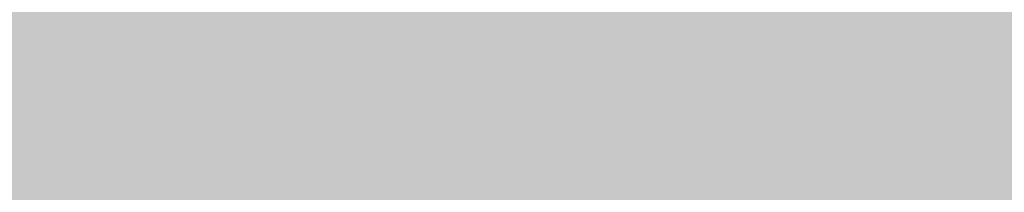
# Model space of a CAD drawing. Units: inches. Extents: x 2091 to 2899, y 967 to 2217.
# Tile 202 of 256: x 2203.18039 to 2203.25707, y 1152.26051 to 1152.27396. Entities that reach past the tile are written whole.
import ezdxf

# ---------------------------------------------------------------- set-up
doc = ezdxf.new("R2010")
doc.units = ezdxf.units.IN
doc.layers.add('A-WALL-PATT', color=141, linetype='Continuous', lineweight=13, true_color=0xadddf7)

msp = doc.modelspace()

# ---------------------------------------------------------------- hatches: boundary and pattern name
at = {"layer": 'A-WALL-PATT'}
h = msp.add_hatch(color=256, dxfattribs=at)
h.dxf.hatch_style = 1
h.paths.add_polyline_path([(2803.143603, 2050.919059), (2203.143603, 2050.919059), (2203.143603, 1090.919059), (2803.143603, 1090.919059)])
h.paths.add_polyline_path([(2635.79885, 1147.540465), (2674.524052, 1147.540465, 0.376086), (2678.529665, 1152.880202), (2678.529665, 1159.556473, 0.333335), (2674.524319, 1163.561846), (2674.524319, 1163.56185), (2674.524319, 1192.93439), (2635.805971, 1192.93439), (2597.087622, 1192.93439), (2597.087622, 1163.561846, 0.333335), (2593.082276, 1159.556473), (2593.082276, 1152.880202, 0.376086), (2597.087889, 1147.540465)], flags=0)
h.paths.add_polyline_path([(2436.010433, 1278.240778, 0.000483), (2435.952643, 1278.215027, -0.001328), (2435.935625, 1278.111693, -0.001711), (2436.11644, 1278.040758, 0.002185)], flags=0)
h.paths.add_polyline_path([(2794.143603, 1143.419059), (2794.143603, 1347.419059), (2543.370171, 1347.419059), (2543.370171, 1351.919059), (2794.143603, 1351.919059), (2794.143603, 1392.713555), (2793.947398, 1392.713555), (2793.947398, 1473.5369), (2794.143603, 1473.5369), (2794.143603, 1531.919059), (2650.143603, 1531.919059), (2650.143603, 1536.419059), (2794.143603, 1536.419059), (2794.143603, 1692.419059), (2609.375609, 1692.419059), (2609.375609, 1644.419059), (2604.875609, 1644.419059), (2604.875609, 1744.919059), (2609.375609, 1744.919059), (2609.375609, 1696.919059), (2794.143603, 1696.919059), (2794.143603, 1780.919059), (2609.643603, 1780.919059), (2493.875609, 1780.919059), (2493.875609, 1785.419059), (2609.643603, 1785.419059), (2794.143603, 1785.419059), (2794.143603, 1847.938821), (2793.951222, 1847.938821), (2793.951222, 1928.762166), (2794.143603, 1928.762166), (2794.143603, 1941.419059), (2614.143603, 1941.419059), (2614.143603, 1821.419059), (2609.643603, 1821.419059), (2609.643603, 1941.419059), (2392.143603, 1941.419059), (2392.143603, 1819.919059), (2387.643603, 1819.919059), (2387.643603, 1941.419059), (2212.143603, 1941.419059), (2212.143603, 1783.919059), (2392.143603, 1783.919059), (2392.143603, 1780.919059), (2212.143603, 1780.919059), (2212.143603, 1629.419059), (2387.643603, 1629.419059), (2387.643603, 1744.919059), (2392.143603, 1744.919059), (2392.143603, 1627.919059), (2317.143603, 1627.919059), (2317.143603, 1551.419059), (2317.143603, 1536.419059), (2459.383591, 1536.419059), (2459.383591, 1602.39648), (2463.883591, 1602.39648), (2463.883591, 1531.919059), (2456.643603, 1531.919059), (2456.643603, 1529.919059), (2452.143603, 1529.919059), (2452.143603, 1531.919059), (2312.643603, 1531.919059), (2312.643603, 1551.419059), (2306.143603, 1551.419059), (2306.143603, 1555.919059), (2308.143603, 1555.919059), (2308.143603, 1551.419059), (2312.643603, 1551.419059), (2312.643603, 1627.919059), (2212.143603, 1627.919059), (2212.143603, 1555.919059), (2270.143603, 1555.919059), (2270.143603, 1551.419059), (2212.143603, 1551.419059), (2212.143603, 1351.919059), (2272.143603, 1351.919059), (2272.143603, 1347.419059), (2212.143603, 1347.419059), (2212.143603, 1275.419059), (2308.143603, 1275.419059), (2308.143603, 1351.919059), (2452.143603, 1351.919059), (2452.143603, 1493.919059), (2456.643603, 1493.919059), (2456.643603, 1347.419059), (2312.643603, 1347.419059), (2312.643603, 1270.919059), (2212.143603, 1270.919059), (2212.143603, 1099.919059), (2281.237523, 1099.919059), (2282.871041, 1110.913803), (2282.008341, 1116.996603), (2278.557741, 1121.420403), (2268.205641, 1128.056203), (2272.087641, 1128.056203), (2273.812941, 1131.927003), (2279.420341, 1134.691903), (2285.027841, 1135.244903), (2287.615841, 1137.456803), (2288.047141, 1138.009803), (2289.341141, 1140.774703), (2291.066541, 1139.668703), (2292.360541, 1135.244903), (2295.379841, 1136.903803), (2296.242541, 1135.797903), (2297.105241, 1133.033003), (2300.124641, 1138.009803), (2303.143941, 1138.009803), (2304.437941, 1135.797903), (2303.143941, 1133.586003), (2306.594641, 1134.691903), (2307.888741, 1133.033003), (2310.908041, 1135.244903), (2313.927441, 1134.138903), (2315.62686, 1132.427102), (2308.320041, 1117.549603), (2290.203841, 1109.807903), (2288.909841, 1103.172103), (2289.272309, 1099.919059), (2434.918227, 1099.919059), (2431.593227, 1124.788059), (2429.930227, 1169.553059), (2430.927185, 1240.519694), (2435.658926, 1238.186126), (2437.135227, 1196.554059), (2438.798227, 1143.973059), (2442.678227, 1111.998059), (2446.558227, 1099.919059), (2794.143603, 1099.919059), (2794.143603, 1138.919059), (2548.032447, 1138.919059), (2548.032447, 1143.419059), (2548.032447, 1148.819059), (2546.668457, 1148.031559), (2528.685692, 1179.178622, 0.256256), (2512.032447, 1148.819059), (2512.032447, 1143.419059), (2512.032447, 1138.919059), (2507.532447, 1138.919059), (2507.532447, 1143.419059), (2507.532447, 1148.819059, 0.256256), (2490.879202, 1179.178622), (2472.896437, 1148.031559), (2471.532447, 1148.819059), (2471.532447, 1143.419059), (2467.032447, 1143.419059), (2467.032447, 1269.945786, 0.039061), (2460.909987, 1273.580059), (2467.032447, 1273.580059), (2467.032447, 1286.325364, 0.014511), (2465.216194, 1286.761905), (2467.032447, 1287.052576), (2467.032447, 1323.419059), (2471.532447, 1323.419059), (2471.532447, 1148.819059), (2489.532447, 1179.995973), (2490.896437, 1179.208473), (2490.879202, 1179.178622, -0.256256), (2507.532447, 1148.819059), (2507.532447, 1143.419059), (2512.032447, 1143.419059), (2512.032447, 1148.819059, -0.256256), (2528.685692, 1179.178622), (2528.668457, 1179.208473), (2530.032447, 1179.995973), (2548.032447, 1148.819059), (2548.032447, 1143.419059)], flags=16)
h.paths.add_polyline_path([(2607.768546, 1200.945083), (2607.768546, 1265.030625), (2597.087622, 1281.052011), (2619.784585, 1281.052011), (2627.795278, 1337.12686), (2635.79885, 1337.12686), (2643.816663, 1337.12686), (2651.827356, 1281.052011), (2674.524319, 1281.052011), (2663.843395, 1265.030625), (2663.843395, 1200.945083), (2635.805971, 1200.945083)], flags=0)
edge = h.paths.add_edge_path(flags=0)
edge.add_ellipse((13303.896215, 1272.998725), major_axis=(-10595.31304, 0.000001), ratio=0.842303870086, start_angle=0.6282372191, end_angle=0.6465540999, ccw=False)
edge.add_ellipse((2711.70045, 1156.852678), major_axis=(2.219769, 0), ratio=0.84230387, start_angle=111.535244, end_angle=180.628237, ccw=False)
edge.add_ellipse((13303.156292, 1272.998725), major_axis=(-10593.026306, 0), ratio=0.842303869544, start_angle=0.5282714718, end_angle=0.6465540971, ccw=False)
edge.add_line((2710.764596, 1175.333295), (2710.129986, 1175.333295))
edge.add_ellipse((2710.129986, 1176.579775), major_axis=(1.479846, 0), ratio=0.84230387, start_angle=180, end_angle=270, ccw=False)
edge.add_line((2708.65014, 1176.579775), (2708.65014, 1200.782914))
edge.add_ellipse((2710.129986, 1200.782914), major_axis=(1.479846, 0), ratio=0.84230387, start_angle=90, end_angle=180, ccw=False)
edge.add_line((2710.129986, 1202.029394), (2710.465075, 1202.029394))
edge.add_ellipse((13303.156292, 1272.998725), major_axis=(-10593.026306, 0), ratio=0.842303869544, start_angle=-0.0902290886, end_angle=0.3838667788, ccw=False)
edge.add_ellipse((2710.129986, 1290.927031), major_axis=(-1.479846, 0), ratio=0.84230387, start_angle=0, end_angle=90, ccw=False)
edge.add_line((2708.65014, 1290.927031), (2708.65014, 1315.13017))
edge.add_ellipse((2710.129986, 1315.13017), major_axis=(-1.479846, 0), ratio=0.84230387, start_angle=-90, end_angle=0, ccw=False)
edge.add_line((2710.129986, 1316.37665), (2710.706314, 1316.37665))
edge.add_ellipse((3238.40172, 1296.289566), major_axis=(528.234, 0), ratio=0.8423038695, start_angle=176.34957241, end_angle=177.82004969, ccw=False)
edge.add_ellipse((2775.063043, 1071.450696), major_axis=(313.307761, 0), ratio=0.8423038695, start_angle=102.12596555, end_angle=103.78052899, ccw=False)
edge.add_ellipse((2775.063043, 1078.305698), major_axis=(-305.302891, 0), ratio=0.8423038695, start_angle=-79.790461, end_angle=-77.55537271, ccw=False)
edge.add_ellipse((2695.141767, 1541.975383), major_axis=(-250.960216, 0), ratio=0.8423038695, start_angle=99.25656601, end_angle=102.55493264)
edge.add_line((2741.410326, 1334.214255), (2747.132545, 1337.378477))
edge.add_ellipse((2747.538616, 1336.857478), major_axis=(-0.739923, 0), ratio=0.8423039, start_angle=270, end_angle=307.93313, ccw=False)
edge.add_ellipse((2747.538616, 1336.857478), major_axis=(-0.739923, 0), ratio=0.8423039, start_angle=232.06687, end_angle=270, ccw=False)
edge.add_line((2747.944687, 1337.378477), (2753.666906, 1334.214255))
edge.add_ellipse((2799.935466, 1541.975383), major_axis=(250.960216, 0), ratio=0.8423038695, start_angle=257.44506736, end_angle=260.74343399)
edge.add_ellipse((2720.014189, 1078.305698), major_axis=(305.302891, 0), ratio=0.8423038695, start_angle=77.55537271, end_angle=79.790461, ccw=False)
edge.add_ellipse((2720.014189, 1071.450696), major_axis=(-313.307761, 0), ratio=0.8423038695, start_angle=256.21947101, end_angle=257.87403445, ccw=False)
edge.add_ellipse((2256.675512, 1296.289566), major_axis=(-528.234, 0), ratio=0.8423038695, start_angle=182.17995031, end_angle=183.65042759, ccw=False)
edge.add_line((2784.370918, 1316.37665), (2784.947247, 1316.37665))
edge.add_ellipse((2784.947247, 1315.13017), major_axis=(1.479846, 0), ratio=0.84230387, start_angle=0, end_angle=90, ccw=False)
edge.add_line((2786.427093, 1315.13017), (2786.427093, 1290.927031))
edge.add_ellipse((2784.947247, 1290.927031), major_axis=(1.479846, 0), ratio=0.84230387, start_angle=270, end_angle=360, ccw=False)
edge.add_ellipse((-7808.07906, 1272.998725), major_axis=(10593.026306, 0), ratio=0.842303869544, start_angle=-0.3838667788, end_angle=0.0902290886, ccw=False)
edge.add_line((2784.612157, 1202.029394), (2784.947247, 1202.029394))
edge.add_ellipse((2784.947247, 1200.782914), major_axis=(1.479846, 0), ratio=0.84230387, start_angle=0, end_angle=90, ccw=False)
edge.add_line((2786.427093, 1200.782914), (2786.427093, 1176.579775))
edge.add_ellipse((2784.947247, 1176.579775), major_axis=(-1.479846, 0), ratio=0.84230387, start_angle=90, end_angle=180, ccw=False)
edge.add_line((2784.947247, 1175.333295), (2784.312636, 1175.333295))
edge.add_ellipse((-7808.07906, 1272.998725), major_axis=(10593.026306, 0), ratio=0.842303869544, start_angle=-0.6186431963, end_angle=-0.5282714718, ccw=False)
edge.add_ellipse((2783.376783, 1156.852678), major_axis=(-2.219769, 0), ratio=0.84230387, start_angle=179.371763, end_angle=248.464757, ccw=False)
edge.add_ellipse((-7808.818983, 1272.998725), major_axis=(-10595.31304, 0.000004), ratio=0.842303865762, start_angle=179.3534459226, end_angle=179.3717628034, ccw=False)
edge.add_ellipse((2780.297303, 1153.500793), major_axis=(-5.246426, 0), ratio=0.84230387, start_angle=90, end_angle=179.353446, ccw=False)
edge.add_line((2780.297303, 1149.081708), (2714.77993, 1149.081708))
edge.add_ellipse((2714.77993, 1153.500793), major_axis=(5.246426, 0), ratio=0.84230387, start_angle=180.646554, end_angle=270, ccw=False)
edge = h.paths.add_edge_path(flags=0)
edge.add_line((2718.187367, 1151.007833), (2718.187367, 1170.472364))
edge.add_ellipse((2721.14706, 1170.472364), major_axis=(-2.959692, 0), ratio=0.84230387, start_angle=-90, end_angle=0, ccw=False)
edge.add_line((2721.14706, 1172.965324), (2773.930173, 1172.965324))
edge.add_ellipse((2773.930173, 1170.472364), major_axis=(-2.959692, 0), ratio=0.84230387, start_angle=180, end_angle=270, ccw=False)
edge.add_line((2776.889865, 1170.472364), (2776.889865, 1151.007833))
edge.add_line((2776.889865, 1151.007833), (2718.187367, 1151.007833))
edge = h.paths.add_edge_path(flags=0)
edge.add_line((2718.187367, 1180.23415), (2718.187367, 1199.057834))
edge.add_ellipse((2747.538616, 1320.39864), major_axis=(147.017924, 0), ratio=0.8423038695, start_angle=256.40186531, end_angle=283.59813469)
edge.add_line((2776.889865, 1199.057834), (2776.889865, 1180.23415))
edge.add_ellipse((2747.538616, 1301.574956), major_axis=(147.017924, 0), ratio=0.8423038695, start_angle=256.40186531, end_angle=283.59813469, ccw=False)
edge = h.paths.add_edge_path(flags=0)
edge.add_ellipse((13303.156292, 1272.998725), major_axis=(-10591.54646, 0), ratio=0.842303869555, start_angle=0.0555943135, end_angle=0.3777641939, ccw=False)
edge.add_line((2711.616859, 1262.72171), (2715.667408, 1249.495396))
edge.add_ellipse((6413.891963, 1241.691919), major_axis=(-3698.236159, 0), ratio=0.84230386955, start_angle=-0.120897369, end_angle=0.364076349)
edge.add_line((2715.761038, 1218.192455), (2711.934307, 1203.167361))
edge = h.paths.add_edge_path(flags=0)
edge.add_line((2718.187367, 1251.074566), (2716.002485, 1267.450435))
edge.add_ellipse((2742.151175, 1202.18954), major_axis=(81.772585, 0), ratio=0.84230387, start_angle=94.27742096, end_angle=111.8349538, ccw=False)
edge.add_line((2737.009748, 1270.930626), (2758.067484, 1270.930626))
edge.add_ellipse((2752.926058, 1202.18954), major_axis=(81.772585, 0), ratio=0.84230387, start_angle=68.1650462, end_angle=85.72257904, ccw=False)
edge.add_line((2779.074747, 1267.450435), (2776.889865, 1251.074566))
edge.add_ellipse((2750.338059, 1187.885356), major_axis=(79.579664, 0), ratio=0.84230387, start_angle=67.20808512, end_angle=85.1299304)
edge.add_line((2756.034656, 1254.743656), (2739.042576, 1254.743656))
edge.add_ellipse((2744.739174, 1187.885356), major_axis=(79.579664, 0), ratio=0.84230387, start_angle=94.8700696, end_angle=112.79191488)
edge = h.paths.add_edge_path(flags=0)
edge.add_line((2783.142926, 1203.167361), (2779.316194, 1218.192455))
edge.add_ellipse((-918.81473, 1241.691919), major_axis=(3698.236159, 0), ratio=0.84230386955, start_angle=-0.364076349, end_angle=0.120897369)
edge.add_line((2779.409825, 1249.495396), (2783.460373, 1262.72171))
edge.add_ellipse((-7808.07906, 1272.998725), major_axis=(-10591.54646, 0), ratio=0.84230386954, start_angle=179.6222358061, end_angle=179.9444056865, ccw=False)
edge = h.paths.add_edge_path(flags=0)
edge.add_ellipse((2734.200892, 1286.69044), major_axis=(-0.356609, 6.340078), ratio=0.60383358, start_angle=89.0020143, end_angle=253.657408, ccw=False)
edge.add_line((2730.369001, 1286.541806), (2730.369001, 1301.35198))
edge.add_line((2730.369001, 1301.35198), (2735.913311, 1305.214803))
edge.add_ellipse((2736.384917, 1304.734561), major_axis=(0.739923, 0), ratio=0.8423039, start_angle=90, end_angle=134.480211, ccw=False)
edge.add_line((2736.384917, 1305.357801), (2738.032783, 1305.357801))
edge.add_line((2738.032783, 1305.357801), (2738.032783, 1307.707927))
edge.add_ellipse((2794.201642, 1307.707927), major_axis=(56.168859, 0), ratio=0.84230387, start_angle=150.5614304, end_angle=180, ccw=False)
edge.add_ellipse((2700.875591, 1307.707927), major_axis=(-56.168859, 0), ratio=0.84230387, start_angle=180, end_angle=209.4385696, ccw=False)
edge.add_line((2757.04445, 1307.707927), (2757.04445, 1305.357801))
edge.add_line((2757.04445, 1305.357801), (2758.692316, 1305.357801))
edge.add_ellipse((2758.692316, 1304.734561), major_axis=(-0.739923, 0), ratio=0.8423039, start_angle=225.519789, end_angle=270, ccw=False)
edge.add_line((2759.163922, 1305.214803), (2764.708231, 1301.35198))
edge.add_line((2764.708231, 1301.35198), (2764.708231, 1286.541806))
edge.add_ellipse((2760.87634, 1286.69044), major_axis=(0.356609, 6.340078), ratio=0.60383358, start_angle=106.342592, end_angle=270.9979857, ccw=False)
edge.add_line((2757.04445, 1285.79709), (2757.04445, 1307.707927))
edge.add_ellipse((2700.875591, 1307.707927), major_axis=(-56.168859, 0), ratio=0.84230387, start_angle=180, end_angle=209.4385696)
edge.add_ellipse((2794.201642, 1307.707927), major_axis=(56.168859, 0), ratio=0.84230387, start_angle=150.5614304, end_angle=180)
edge.add_line((2738.032783, 1307.707927), (2738.032783, 1285.79709))
h.paths.add_polyline_path([(2417.812273, 1104.449704), (2413.492273, 1102.529704), (2410.612273, 1103.969704), (2409.172273, 1106.369704), (2407.252273, 1107.329704), (2406.292273, 1109.729704), (2405.332273, 1114.049704), (2405.332273, 1117.889704), (2406.292273, 1120.129704), (2407.252273, 1119.809704), (2408.848322, 1118.327658), (2410.173945, 1119.42417), (2410.211273, 1120.405704), (2411.040731, 1121.419054), (2410.699273, 1119.858704), (2410.173945, 1119.42417), (2410.088452, 1117.176109), (2411.132836, 1116.206324), (2413.972273, 1119.329704), (2416.852273, 1120.769704), (2416.869721, 1120.798784), (2417.035071, 1119.405116), (2417.896213, 1118.143384), (2418.292273, 1118.369704), (2419.544447, 1120.039269), (2419.360915, 1118.387487), (2419.032108, 1119.356151), (2418.398939, 1118.511926), (2419.252273, 1114.529704), (2418.794091, 1107.198795)], flags=0)
h.paths.add_polyline_path([(2508.870171, 1347.419059), (2508.370171, 1347.419059), (2508.370171, 1351.919059), (2508.870171, 1351.919059)], flags=0)
h.paths.add_polyline_path([(2473.370171, 1347.419059), (2472.370171, 1347.419059), (2467.870171, 1347.419059), (2467.870171, 1455.419059), (2472.370171, 1455.419059), (2472.370171, 1352.419059), (2473.370171, 1352.419059)], flags=0)
h.paths.add_polyline_path([(2352.106244, 1217.446197), (2349.226244, 1218.886197), (2347.786244, 1221.286197), (2345.866244, 1222.246197), (2344.906244, 1224.646197), (2343.946244, 1228.966197), (2343.946244, 1232.806197), (2344.906244, 1235.046197), (2345.866244, 1234.726197), (2347.462293, 1233.244152), (2348.787916, 1234.340663), (2348.825244, 1235.322197), (2349.654702, 1236.335547), (2349.313244, 1234.775197), (2348.787916, 1234.340663), (2348.702423, 1232.092603), (2349.746807, 1231.122817), (2352.586244, 1234.246197), (2355.466244, 1235.686197), (2355.483692, 1235.715277), (2355.649043, 1234.321609), (2356.510185, 1233.059877), (2356.906244, 1233.286197), (2358.158418, 1234.955762), (2357.974887, 1233.30398), (2357.646079, 1234.272644), (2357.012911, 1233.428419), (2357.866244, 1229.446197), (2357.408062, 1222.115288), (2356.426244, 1219.366197)], flags=0)
h.paths.add_polyline_path([(2348.2968, 1112.22442), (2347.0138, 1112.31042), (2345.5298, 1114.12742), (2345.7318, 1115.85842), (2346.8118, 1116.98242), (2346.8118, 1114.64642), (2345.8668, 1114.21442), (2346.8798, 1114.30042)], flags=0)
h.paths.add_polyline_path([(2347.0138, 1110.92642), (2346.2718, 1110.49342), (2346.6098, 1111.18642)], flags=0)
h.paths.add_polyline_path([(2345.8668, 1118.19442), (2345.5298, 1117.32942), (2343.7078, 1118.02142), (2344.3828, 1118.62642)], flags=0)
h.paths.add_polyline_path([(2346.6768, 1109.28242), (2346.0698, 1108.07142), (2345.8668, 1110.06142)], flags=0)
h.paths.add_polyline_path([(2345.0568, 1119.75142), (2343.6398, 1119.75142), (2343.9778, 1121.13542)], flags=0)
h.paths.add_polyline_path([(2345.2598, 1116.55042), (2345.1248, 1115.85842), (2344.9218, 1115.68542), (2344.7198, 1116.37742)], flags=0)
h.paths.add_polyline_path([(2345.6648, 1112.31042), (2345.4618, 1111.53242), (2344.0448, 1111.96442), (2344.6518, 1112.57042)], flags=0)
h.paths.add_polyline_path([(2345.1918, 1113.34942), (2344.4498, 1113.86842), (2344.7198, 1114.38742)], flags=0)
h.paths.add_polyline_path([(2344.6518, 1116.80942), (2344.1798, 1115.68542), (2344.6518, 1115.33942), (2343.9098, 1114.90642), (2343.0328, 1115.94442), (2343.6398, 1116.46342)], flags=0)
h.paths.add_polyline_path([(2345.8668, 1106.68642), (2344.9898, 1105.56242), (2344.5168, 1106.60042)], flags=0)
h.paths.add_polyline_path([(2344.8548, 1110.06142), (2344.5168, 1109.28242), (2344.1128, 1109.71542)], flags=0)
h.paths.add_polyline_path([(2344.0448, 1113.52242), (2343.4378, 1113.08942), (2342.7628, 1113.95442)], flags=0)
h.paths.add_polyline_path([(2344.3148, 1111.01242), (2342.9648, 1110.32042), (2342.9648, 1111.09942)], flags=0)
h.paths.add_polyline_path([(2345.1248, 1104.69742), (2344.5848, 1103.74542), (2344.4498, 1104.26442)], flags=0)
h.paths.add_polyline_path([(2342.8298, 1121.22242), (2341.7498, 1120.53042), (2340.5358, 1121.04942), (2340.1308, 1121.82842), (2340.6708, 1122.95242), (2341.1428, 1121.82842), (2341.6148, 1122.00142)], flags=0)
h.paths.add_polyline_path([(2342.9648, 1119.75142), (2343.0328, 1118.45342), (2342.0878, 1118.02142), (2342.0198, 1119.49142)], flags=0)
h.paths.add_polyline_path([(2342.6948, 1116.89642), (2341.9528, 1116.63642), (2342.0198, 1117.32942)], flags=0)
h.paths.add_polyline_path([(2343.0328, 1112.22442), (2342.0198, 1111.79142), (2341.5478, 1112.22442), (2342.3578, 1113.34942)], flags=0)
h.paths.add_polyline_path([(2343.7748, 1104.43742), (2342.6278, 1102.88042), (2342.6948, 1104.61042), (2343.4378, 1105.12942)], flags=0)
h.paths.add_polyline_path([(2342.0198, 1115.07942), (2340.8058, 1115.51242), (2340.9408, 1116.37742)], flags=0)
h.paths.add_polyline_path([(2341.4808, 1120.09742), (2341.4808, 1119.40542), (2341.0758, 1119.57842), (2341.1428, 1120.09742)], flags=0)
h.paths.add_polyline_path([(2341.8178, 1114.47342), (2340.9408, 1113.08942), (2340.8058, 1114.56042)], flags=0)
h.paths.add_polyline_path([(2341.1428, 1118.54042), (2340.9408, 1116.98242), (2339.0508, 1117.67542), (2339.0508, 1118.62642)], flags=0)
h.paths.add_polyline_path([(2342.6948, 1101.66842), (2341.9528, 1101.84142), (2342.5598, 1102.36142)], flags=0)
h.paths.add_polyline_path([(2340.3328, 1119.66542), (2338.4438, 1119.57842), (2337.9038, 1120.35742), (2339.6578, 1120.61642)], flags=0)
h.paths.add_polyline_path([(2340.3328, 1115.33942), (2340.0628, 1113.69542), (2339.3878, 1115.33942)], flags=0)
h.paths.add_polyline_path([(2341.8178, 1103.83142), (2341.5478, 1102.88042), (2341.1428, 1103.65842)], flags=0)
h.paths.add_polyline_path([(2339.0508, 1122.86642), (2337.2958, 1121.82842), (2337.0938, 1123.12542), (2337.7688, 1123.81842)], flags=0)
h.paths.add_polyline_path([(2339.1178, 1121.74142), (2338.8478, 1121.22242), (2338.1738, 1121.04942), (2338.3758, 1121.56842)], flags=0)
h.paths.add_polyline_path([(2339.1858, 1119.31942), (2338.6458, 1118.71342), (2338.2408, 1118.10742), (2338.2408, 1118.88642)], flags=0)
h.paths.add_polyline_path([(2341.1428, 1101.92842), (2340.6028, 1101.23642), (2340.0628, 1101.84142), (2340.6028, 1102.36142)], flags=0)
h.paths.add_polyline_path([(2337.6338, 1117.76142), (2336.6208, 1118.28042), (2337.2958, 1118.97242)], flags=0)
h.paths.add_polyline_path([(2336.8238, 1119.57842), (2334.7988, 1118.97242), (2335.2038, 1120.35742), (2336.5538, 1120.87642)], flags=0)
h.paths.add_polyline_path([(2339.1178, 1100.45742), (2337.3638, 1100.54342), (2336.7558, 1101.23642)], flags=0)
h.paths.add_polyline_path([(2336.3508, 1122.43342), (2336.0138, 1121.91442), (2334.9338, 1122.43342), (2334.5288, 1123.47142), (2335.7438, 1122.77942)], flags=0)
h.paths.add_polyline_path([(2334.7318, 1120.87642), (2334.2588, 1120.35742), (2334.0568, 1120.78942), (2334.5968, 1121.30842)], flags=0)
h.paths.add_polyline_path([(2334.4618, 1122.17442), (2332.5718, 1121.30842), (2331.3568, 1122.17442), (2332.0998, 1122.86642)], flags=0)
h.paths.add_polyline_path([(2334.2588, 1118.54042), (2333.3818, 1118.45342), (2333.6518, 1119.31942)], flags=0)
h.paths.add_polyline_path([(2335.5418, 1102.27442), (2334.1918, 1102.62042), (2335.2718, 1103.31242)], flags=0)
h.paths.add_polyline_path([(2332.7068, 1119.66542), (2331.6948, 1120.44342), (2332.5048, 1120.78942)], flags=0)
h.paths.add_polyline_path([(2334.7318, 1101.14942), (2333.5168, 1101.58242), (2333.9888, 1101.75542)], flags=0)
h.paths.add_polyline_path([(2332.6398, 1116.63642), (2331.0868, 1116.29042), (2331.9648, 1118.19442)], flags=0)
h.paths.add_polyline_path([(2330.7498, 1121.56842), (2330.2768, 1120.27042), (2328.5228, 1119.31942), (2328.9948, 1121.04942)], flags=0)
h.paths.add_polyline_path([(2330.7498, 1118.62642), (2330.0078, 1117.50242), (2329.8728, 1118.02142)], flags=0)
h.paths.add_polyline_path([(2332.0998, 1102.36142), (2330.5468, 1102.01442), (2331.6948, 1102.96642)], flags=0)
h.paths.add_polyline_path([(2329.5348, 1113.60842), (2329.0628, 1112.31042), (2328.5898, 1113.34942)], flags=0)
h.paths.add_polyline_path([(2328.3878, 1117.84842), (2327.5098, 1116.55042), (2327.1728, 1117.76142)], flags=0)
h.paths.add_polyline_path([(2329.7378, 1106.51342), (2329.5348, 1105.30242), (2328.2528, 1106.08142)], flags=0)
h.paths.add_polyline_path([(2328.6578, 1114.38742), (2328.0498, 1114.12742), (2328.3198, 1114.90642)], flags=0)
h.paths.add_polyline_path([(2328.3198, 1112.22442), (2327.1058, 1112.13742), (2326.7008, 1112.65642)], flags=0)
h.paths.add_polyline_path([(2326.9028, 1115.25242), (2326.7008, 1114.12742), (2325.2158, 1113.60842), (2326.0928, 1115.33942)], flags=0)
h.paths.add_polyline_path([(2326.6328, 1108.33042), (2326.0928, 1107.37942), (2325.8908, 1108.50342), (2326.4978, 1109.10942)], flags=0)
h.paths.add_polyline_path([(2615.143603, 1531.919059), (2609.643603, 1531.919059), (2609.643603, 1620.419059), (2614.143603, 1620.419059), (2614.143603, 1536.419059), (2615.143603, 1536.419059)], flags=0)
h.paths.add_polyline_path([(2545.143603, 1563.419059), (2464.143603, 1563.419059), (2464.143603, 1632.419059), (2509.143603, 1632.419059), (2509.143603, 1627.919059), (2509.143603, 1603.919059), (2468.643603, 1603.919059), (2468.643603, 1567.919059), (2540.643603, 1567.919059), (2540.643603, 1591.919059), (2545.143603, 1591.919059)], flags=0)
h.paths.add_polyline_path([(2388.969048, 1549.985735), (2357.434181, 1549.985735), (2357.434181, 1623.360778), (2399.362777, 1623.360778), (2435.689465, 1623.360778), (2435.592547, 1602.559273), (2435.592547, 1602.39648), (2388.969048, 1602.39648)], flags=0)
h.paths.add_polyline_path([(2388.880628, 1555.809151), (2374.904429, 1555.809151), (2374.904429, 1600.571564), (2374.904429, 1615.457645), (2406.350877, 1615.457645), (2406.350877, 1618.939431), (2412.174293, 1615.457645), (2406.350877, 1611.97586), (2406.350877, 1615.457645), (2388.880628, 1615.457645)], flags=0)
h.paths.add_polyline_path([(2568.875609, 1644.419059), (2453.375609, 1644.419059), (2453.375609, 1785.419059), (2457.875609, 1785.419059), (2457.875609, 1648.919059), (2568.875609, 1648.919059)], flags=0)
h.paths.add_polyline_path([(2212.143603, 1945.919059), (2212.143603, 2041.919059), (2794.143603, 2041.919059), (2794.143603, 1945.919059)], flags=16)
h.paths.add_polyline_path([(2271.082728, 1964.317238), (2776.852968, 1964.317238), (2776.852968, 2037.169623), (2271.082728, 2037.169623)], flags=8)
h.paths.add_polyline_path([(2380.649285, 1536.824144), (2461.040809, 1536.824144), (2461.040809, 1554.652587), (2380.649285, 1554.652587)], flags=8)
h.paths.add_polyline_path([(2240.755709, 1609.725451), (2309.185829, 1609.725451), (2309.185829, 1617.698204), (2240.755709, 1617.698204)], flags=8)
h.paths.add_polyline_path([(2212.677255, 1313.504102), (2282.59152, 1313.504102), (2282.59152, 1322.745239), (2212.677255, 1322.745239)], flags=8)
h.paths.add_polyline_path([(2457.111976, 1114.778574), (2558.481581, 1114.778574), (2558.481581, 1142.219682), (2457.111976, 1142.219682)], flags=8)
h.paths.add_polyline_path([(2473.442337, 1273.010067), (2604.641226, 1273.010067), (2604.641226, 1318.346935), (2473.442337, 1318.346935)], flags=8)
h.paths.add_polyline_path([(2638.876302, 1626.977432), (2684.250367, 1627.976738), (2684.038483, 1637.597494), (2638.664417, 1636.598188)], flags=8)
h.paths.add_polyline_path([(2537.590554, 1453.793447), (2628.389547, 1453.793447), (2628.389547, 1475.344811), (2537.590554, 1475.344811)], flags=8)
h.paths.add_polyline_path([(2504.137638, 1714.632397), (2554.647187, 1714.632397), (2554.647187, 1730.237712), (2504.137638, 1730.237712)], flags=8)
h.paths.add_polyline_path([(2487.501181, 1575.651872), (2535.097121, 1575.651872), (2535.097121, 1598.377646), (2487.501181, 1598.377646)], flags=8)
h.paths.add_polyline_path([(2709.0994, 1735.710278), (2740.016601, 1735.710278), (2740.016601, 1749.937641), (2709.0994, 1749.937641)], flags=8)
h.paths.add_polyline_path([(2442.438424, 1792.171657), (2564.728835, 1792.171657), (2564.728835, 1842.000163), (2442.438424, 1842.000163)], flags=8)
h.paths.add_polyline_path([(2655.815801, 1809.644076), (2789.520142, 1806.693796), (2790.084977, 1832.291638), (2656.380635, 1835.241918)], flags=8)
h.paths.add_polyline_path([(2234.842697, 1797.720143), (2368.592851, 1794.768852), (2369.160718, 1820.504132), (2235.410564, 1823.455423)], flags=8)
h.paths.add_polyline_path([(2245.138466, 1644.006335), (2398.427733, 1640.6239), (2398.994842, 1666.32482), (2245.705575, 1669.707255)], flags=8)
h.paths.add_polyline_path([(2306.142847, 1431.168519), (2413.768314, 1428.793687), (2414.333148, 1454.391529), (2306.707682, 1456.76636)], flags=8)
h.paths.add_polyline_path([(2306.834582, 1458.233145), (2393.380484, 1456.323449), (2393.932808, 1481.354358), (2307.386907, 1483.264054)], flags=8)

doc.saveas('drawing.dxf')
